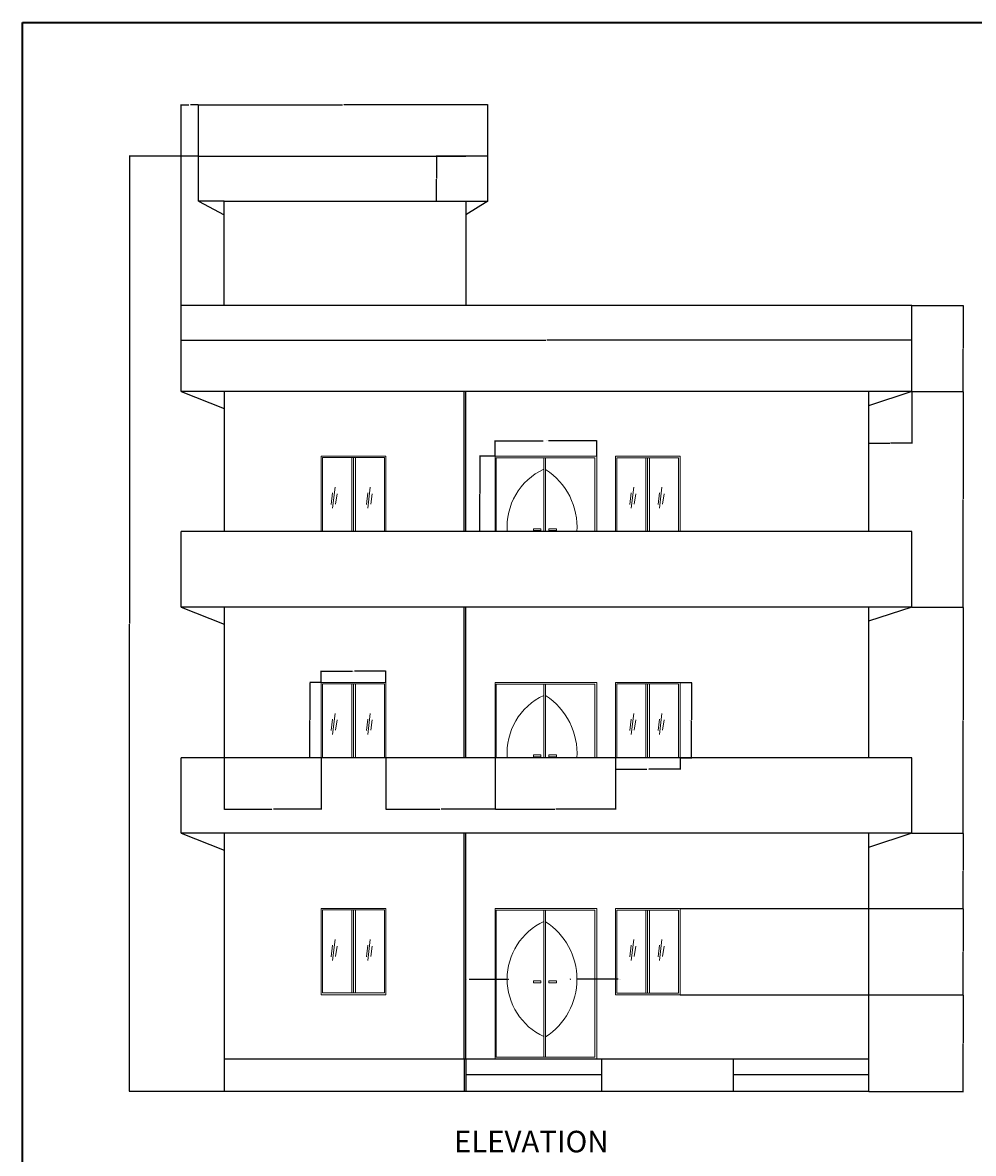
# Model space of a CAD drawing. Units: inches. Extents: x 1832 to 2989, y 1644 to 2902.
# Tile 7 of 8: x 1832 to 2361, y 2272 to 2902. Entities that reach past the tile are written whole.
import ezdxf

# ---------------------------------------------------------------- set-up
doc = ezdxf.new("R2010")
doc.units = ezdxf.units.IN
for name, color, linetype, lineweight in [('A-ANNO-DIMS', 2, 'Continuous', 18), ('A-ANNO-TEXT', 7, 'Continuous', 25), ('A-ANNO-TTLB', 7, 'Continuous', 35), ('A-ELEV', 7, 'Continuous', 25), ('A-ELEV-DOOR', 3, 'Continuous', 18), ('A-ELEV-GLAZ', 4, 'Continuous', 18)]:
    doc.layers.add(name, color=color, linetype=linetype, lineweight=lineweight)
doc.styles.get("Standard").update_dxf_attribs({"font": 'arial.ttf'})
doc.dimstyles.get("Standard").update_dxf_attribs({"dimtxt": 0.18, "dimasz": 0.18, "dimexe": 0.18, "dimexo": 0.0625, "dimgap": 0.09, "dimtad": 0, "dimtih": 1, "dimtoh": 1, "dimdec": 4, "dimzin": 0, "dimdsep": 46, "dimtxsty": 'Standard', "dimcen": 0.09, "dimadec": 0, "dimazin": 0, "dimtfac": 1, "dimtdec": 4, "dimtofl": 0, "dimtmove": 0, "dimatfit": 3, "dimfxl": 1, "dimtolj": 1, "dimtzin": 0, "dimarcsym": 0})

# ---------------------------------------------------------------- blocks, each defined once
blk = doc.blocks.new('WIN-ELEV-UPPER-LEFT')
for p, q in [((0, 42), (0, 0)), ((36, 42), (0, 42)), ((17.96, 41.22), (16.96, 41.22)), ((16.96, 41.22), (16.96, 0)), ((17.96, 41.22), (17.96, 0)), ((18.96, 41.22), (17.96, 41.22)), ((18.96, 0), (18.96, 41.22)), ((36, 42), (36, 0)), ((6.3, 21.56), (5.52, 15.16)), ((7.63, 24.74), (6.29, 13.04)), ((8.79, 21.07), (7.93, 15.34)), ((25.93, 21.56), (25.15, 15.16)), ((27.26, 24.74), (25.92, 13.04)), ((28.42, 21.07), (27.56, 15.34))]:
    blk.add_line(p, q)
blk.add_lwpolyline([(0.65, 0), (0.65, 41.22), (35.27, 41.22), (35.27, 0)])
blk = doc.blocks.new('DOOR-ELEV-UPPER')
for p, q in [((0, 42), (0, 0)), ((56.64, 42), (0, 42)), ((27.18, 0), (27.18, 41.04)), ((28.18, 41.04), (28.18, 0)), ((56.64, 42), (56.64, 0))]:
    blk.add_line(p, q)
blk.add_lwpolyline([(0.72, 0), (0.72, 41.04), (55.64, 41.04), (55.64, 0)])
for points in [[(21.46, 1.64), (25.62, 1.64), (25.62, 0.56), (21.46, 0.56)], [(30.06, 1.64), (34.22, 1.64), (34.22, 0.56), (30.06, 0.56)]]:
    blk.add_lwpolyline(points, close=True)
for centre, radius, start, end in [((42.11, 2.72), 35.37, 114.9672, 184.41429), ((7.59, 2.58), 38.09, 356.10922, 57.26734)]:
    blk.add_arc(centre, radius, start, end)
blk = doc.blocks.new('WIN-ELEV-UPPER-RIGHT')
for p, q in [((0, 42), (0, 0)), ((36, 42), (0, 42)), ((17.93, 41.14), (16.93, 41.14)), ((16.93, 41.14), (16.93, 0)), ((17.93, 41.14), (17.93, 0)), ((18.93, 0), (18.93, 41.14)), ((36, 42), (36, 0)), ((8.84, 21.56), (8.06, 15.16)), ((10.17, 24.74), (8.82, 13.04)), ((11.33, 21.07), (10.47, 15.34)), ((24.59, 21.56), (23.81, 15.16)), ((25.92, 24.74), (24.57, 13.04)), ((27.08, 21.07), (26.22, 15.34))]:
    blk.add_line(p, q)
blk.add_lwpolyline([(0.74, 0), (0.74, 41.14), (35.12, 41.14), (35.12, 0)])
blk = doc.blocks.new('*D61')
at = {"layer": 'A-ANNO-DIMS', "color": 0, "lineweight": -2, "transparency": 16777216}
for p, q in [((1997.98, 2534.31), (1991.56, 2534.31)), ((1991.74, 2534.13), (1991.74, 2513.5)), ((1991.74, 2492.49), (1991.74, 2513.13)), ((1997.98, 2492.31), (1991.56, 2492.31))]:
    blk.add_line(p, q, dxfattribs=at)
at = {"layer": 'A-ANNO-DIMS', "color": 0, "transparency": 16777216}
for points in [[(1991.71, 2534.13), (1991.77, 2534.13), (1991.74, 2534.31)], [(1991.71, 2492.49), (1991.77, 2492.49), (1991.74, 2492.31)]]:
    blk.add_solid(points, dxfattribs=at)
at = {"layer": 'Defpoints', "color": 0, "transparency": 16777216}
for p in [(1991.74, 2534.31), (1998.04, 2534.31), (1998.04, 2492.31)]:
    blk.add_point(p, dxfattribs=at)
at = {"layer": 'A-ANNO-DIMS', "color": 0, "transparency": 16777216, "insert": (1991.74, 2513.31), "char_height": 0.18, "attachment_point": 5}
blk.add_mtext('\\A1;LH WINDOW 42 TYP.', dxfattribs=at)
blk = doc.blocks.new('*D62')
at = {"layer": 'A-ANNO-DIMS', "color": 0, "lineweight": -2, "transparency": 16777216}
for p, q in [((1998.04, 2534.37), (1998.04, 2540.79)), ((1998.22, 2540.61), (2015.51, 2540.61)), ((2033.86, 2540.61), (2016.57, 2540.61)), ((2034.04, 2534.37), (2034.04, 2540.79))]:
    blk.add_line(p, q, dxfattribs=at)
at = {"layer": 'A-ANNO-DIMS', "color": 0, "transparency": 16777216}
for points in [[(1998.22, 2540.64), (1998.22, 2540.58), (1998.04, 2540.61)], [(2033.86, 2540.64), (2033.86, 2540.58), (2034.04, 2540.61)]]:
    blk.add_solid(points, dxfattribs=at)
at = {"layer": 'Defpoints', "color": 0, "transparency": 16777216}
for p in [(2034.04, 2540.61), (1998.04, 2534.31), (2034.04, 2534.31)]:
    blk.add_point(p, dxfattribs=at)
at = {"layer": 'A-ANNO-DIMS', "color": 0, "transparency": 16777216, "insert": (2016.04, 2540.61), "char_height": 0.18, "attachment_point": 5}
blk.add_mtext('\\A1;36 TYP.', dxfattribs=at)
blk = doc.blocks.new('*D63')
at = {"layer": 'A-ANNO-DIMS', "color": 0, "lineweight": -2, "transparency": 16777216}
for p, q in [((2094.8, 2660.37), (2094.8, 2668.99)), ((2094.98, 2668.81), (2121.71, 2668.81)), ((2151.25, 2668.81), (2124.52, 2668.81)), ((2151.43, 2660.37), (2151.43, 2668.99))]:
    blk.add_line(p, q, dxfattribs=at)
at = {"layer": 'A-ANNO-DIMS', "color": 0, "transparency": 16777216}
for points in [[(2094.98, 2668.84), (2094.98, 2668.78), (2094.8, 2668.81)], [(2151.25, 2668.84), (2151.25, 2668.78), (2151.43, 2668.81)]]:
    blk.add_solid(points, dxfattribs=at)
at = {"layer": 'Defpoints', "color": 0, "transparency": 16777216}
for p in [(2151.43, 2668.81), (2094.8, 2660.31), (2151.43, 2660.31)]:
    blk.add_point(p, dxfattribs=at)
at = {"layer": 'A-ANNO-DIMS', "color": 0, "transparency": 16777216, "insert": (2123.12, 2668.81), "char_height": 0.18, "attachment_point": 5}
blk.add_mtext('\\A1;UPPER DOOR 57 TYP.', dxfattribs=at)
blk = doc.blocks.new('*D64')
at = {"layer": 'A-ANNO-DIMS', "color": 0, "lineweight": -2, "transparency": 16777216}
for p, q in [((2094.73, 2660.31), (2086.12, 2660.31)), ((2086.3, 2660.13), (2086.3, 2639.49)), ((2086.3, 2618.49), (2086.3, 2639.13)), ((2094.73, 2618.31), (2086.12, 2618.31))]:
    blk.add_line(p, q, dxfattribs=at)
at = {"layer": 'A-ANNO-DIMS', "color": 0, "transparency": 16777216}
for points in [[(2086.27, 2660.13), (2086.33, 2660.13), (2086.3, 2660.31)], [(2086.27, 2618.49), (2086.33, 2618.49), (2086.3, 2618.31)]]:
    blk.add_solid(points, dxfattribs=at)
at = {"layer": 'Defpoints', "color": 0, "transparency": 16777216}
for p in [(2086.3, 2660.31), (2094.8, 2660.31), (2094.8, 2618.31)]:
    blk.add_point(p, dxfattribs=at)
at = {"layer": 'A-ANNO-DIMS', "color": 0, "transparency": 16777216, "insert": (2086.3, 2639.31), "char_height": 0.18, "attachment_point": 5}
blk.add_mtext('\\A1;42 TYP.', dxfattribs=at)
blk = doc.blocks.new('*D65')
at = {"layer": 'A-ANNO-DIMS', "color": 0, "lineweight": -2, "transparency": 16777216}
for p, q in [((2197.95, 2534.31), (2204.37, 2534.31)), ((2204.19, 2534.13), (2204.19, 2513.5)), ((2204.19, 2492.49), (2204.19, 2513.13)), ((2197.95, 2492.31), (2204.37, 2492.31))]:
    blk.add_line(p, q, dxfattribs=at)
at = {"layer": 'A-ANNO-DIMS', "color": 0, "transparency": 16777216}
for points in [[(2204.16, 2534.13), (2204.22, 2534.13), (2204.19, 2534.31)], [(2204.16, 2492.49), (2204.22, 2492.49), (2204.19, 2492.31)]]:
    blk.add_solid(points, dxfattribs=at)
at = {"layer": 'Defpoints', "color": 0, "transparency": 16777216}
for p in [(2197.89, 2534.31), (2204.19, 2534.31), (2197.89, 2492.31)]:
    blk.add_point(p, dxfattribs=at)
at = {"layer": 'A-ANNO-DIMS', "color": 0, "transparency": 16777216, "insert": (2204.19, 2513.31), "char_height": 0.18, "attachment_point": 5}
blk.add_mtext('\\A1;RH WINDOW 42 TYP.', dxfattribs=at)
blk = doc.blocks.new('*D66')
at = {"layer": 'A-ANNO-DIMS', "color": 0, "lineweight": -2, "transparency": 16777216}
for p, q in [((2161.89, 2492.25), (2161.89, 2485.83)), ((2197.89, 2492.25), (2197.89, 2485.83)), ((2162.07, 2486.01), (2179.36, 2486.01)), ((2197.71, 2486.01), (2180.42, 2486.01))]:
    blk.add_line(p, q, dxfattribs=at)
at = {"layer": 'A-ANNO-DIMS', "color": 0, "transparency": 16777216}
for points in [[(2162.07, 2486.04), (2162.07, 2485.98), (2161.89, 2486.01)], [(2197.71, 2486.04), (2197.71, 2485.98), (2197.89, 2486.01)]]:
    blk.add_solid(points, dxfattribs=at)
at = {"layer": 'Defpoints', "color": 0, "transparency": 16777216}
for p in [(2161.89, 2492.31), (2197.89, 2492.31), (2197.89, 2486.01)]:
    blk.add_point(p, dxfattribs=at)
at = {"layer": 'A-ANNO-DIMS', "color": 0, "transparency": 16777216, "insert": (2179.89, 2486.01), "char_height": 0.18, "attachment_point": 5}
blk.add_mtext('\\A1;36 TYP.', dxfattribs=at)
blk = doc.blocks.new('*D98')
at = {"layer": 'A-ANNO-DIMS', "color": 0, "lineweight": -2, "transparency": 16777216}
for p, q in [((1919.89, 2696.37), (1919.89, 2725.14)), ((1920.07, 2724.96), (2123.1, 2724.96)), ((2326.71, 2724.96), (2123.68, 2724.96)), ((2326.89, 2696.37), (2326.89, 2725.14))]:
    blk.add_line(p, q, dxfattribs=at)
at = {"layer": 'A-ANNO-DIMS', "color": 0, "transparency": 16777216}
for points in [[(1920.07, 2724.99), (1920.07, 2724.93), (1919.89, 2724.96)], [(2326.71, 2724.99), (2326.71, 2724.93), (2326.89, 2724.96)]]:
    blk.add_solid(points, dxfattribs=at)
at = {"layer": 'Defpoints', "color": 0, "transparency": 16777216}
for p in [(2326.89, 2724.96), (1919.89, 2696.31), (2326.89, 2696.31)]:
    blk.add_point(p, dxfattribs=at)
at = {"layer": 'A-ANNO-DIMS', "color": 0, "transparency": 16777216, "insert": (2123.39, 2724.96), "char_height": 0.18, "attachment_point": 5}
blk.add_mtext('\\A1;407', dxfattribs=at)
blk = doc.blocks.new('*D99')
at = {"layer": 'A-ANNO-DIMS', "color": 0, "lineweight": -2, "transparency": 16777216}
for p, q in [((1929.52, 2827.51), (1891.06, 2827.51)), ((1891.24, 2827.33), (1891.24, 2567.09)), ((1891.24, 2306.49), (1891.24, 2566.73)), ((1943.83, 2306.31), (1891.06, 2306.31))]:
    blk.add_line(p, q, dxfattribs=at)
at = {"layer": 'A-ANNO-DIMS', "color": 0, "transparency": 16777216}
for points in [[(1891.21, 2827.33), (1891.27, 2827.33), (1891.24, 2827.51)], [(1891.21, 2306.49), (1891.27, 2306.49), (1891.24, 2306.31)]]:
    blk.add_solid(points, dxfattribs=at)
at = {"layer": 'Defpoints', "color": 0, "transparency": 16777216}
for p in [(1891.24, 2827.51), (1929.58, 2827.51), (1943.89, 2306.31)]:
    blk.add_point(p, dxfattribs=at)
at = {"layer": 'A-ANNO-DIMS', "color": 0, "transparency": 16777216, "insert": (1891.24, 2566.91), "char_height": 0.18, "attachment_point": 5}
blk.add_mtext('\\A1;521.2', dxfattribs=at)
blk = doc.blocks.new('*D100')
at = {"layer": 'A-ANNO-DIMS', "color": 0, "lineweight": -2, "transparency": 16777216}
for p, q in [((1919.89, 2744.37), (1919.89, 2856.34)), ((1920.07, 2856.16), (1924.34, 2856.16)), ((1929.4, 2856.16), (1925.13, 2856.16)), ((1929.58, 2827.57), (1929.58, 2856.34))]:
    blk.add_line(p, q, dxfattribs=at)
at = {"layer": 'A-ANNO-DIMS', "color": 0, "transparency": 16777216}
for points in [[(1920.07, 2856.19), (1920.07, 2856.13), (1919.89, 2856.16)], [(1929.4, 2856.19), (1929.4, 2856.13), (1929.58, 2856.16)]]:
    blk.add_solid(points, dxfattribs=at)
at = {"layer": 'Defpoints', "color": 0, "transparency": 16777216}
for p in [(1929.58, 2856.16), (1929.58, 2827.51), (1919.89, 2744.31)]:
    blk.add_point(p, dxfattribs=at)
at = {"layer": 'A-ANNO-DIMS', "color": 0, "transparency": 16777216, "insert": (1924.74, 2856.16), "char_height": 0.18, "attachment_point": 5}
blk.add_mtext('\\A1;9.692', dxfattribs=at)
blk = doc.blocks.new('*D101')
at = {"layer": 'A-ANNO-DIMS', "color": 0, "lineweight": -2, "transparency": 16777216}
for p, q in [((1929.58, 2827.57), (1929.58, 2856.34)), ((1929.76, 2856.16), (2009.79, 2856.16)), ((2090.59, 2856.16), (2010.56, 2856.16)), ((2090.77, 2827.57), (2090.77, 2856.34))]:
    blk.add_line(p, q, dxfattribs=at)
at = {"layer": 'A-ANNO-DIMS', "color": 0, "transparency": 16777216}
for points in [[(1929.76, 2856.19), (1929.76, 2856.13), (1929.58, 2856.16)], [(2090.59, 2856.19), (2090.59, 2856.13), (2090.77, 2856.16)]]:
    blk.add_solid(points, dxfattribs=at)
at = {"layer": 'Defpoints', "color": 0, "transparency": 16777216}
for p in [(2090.77, 2856.16), (1929.58, 2827.51), (2090.77, 2827.51)]:
    blk.add_point(p, dxfattribs=at)
at = {"layer": 'A-ANNO-DIMS', "color": 0, "transparency": 16777216, "insert": (2010.18, 2856.16), "char_height": 0.18, "attachment_point": 5}
blk.add_mtext('\\A1;161.2', dxfattribs=at)
blk = doc.blocks.new('*D102')
at = {"layer": 'A-ANNO-DIMS', "color": 0, "lineweight": -2, "transparency": 16777216}
for p, q in [((2302.89, 2696.25), (2302.89, 2667.48)), ((2326.89, 2696.25), (2326.89, 2667.48)), ((2303.07, 2667.66), (2314.67, 2667.66)), ((2326.71, 2667.66), (2315.11, 2667.66))]:
    blk.add_line(p, q, dxfattribs=at)
at = {"layer": 'A-ANNO-DIMS', "color": 0, "transparency": 16777216}
for points in [[(2303.07, 2667.69), (2303.07, 2667.63), (2302.89, 2667.66)], [(2326.71, 2667.69), (2326.71, 2667.63), (2326.89, 2667.66)]]:
    blk.add_solid(points, dxfattribs=at)
at = {"layer": 'Defpoints', "color": 0, "transparency": 16777216}
for p in [(2302.89, 2696.31), (2326.89, 2696.31), (2302.89, 2667.66)]:
    blk.add_point(p, dxfattribs=at)
at = {"layer": 'A-ANNO-DIMS', "color": 0, "transparency": 16777216, "insert": (2314.89, 2667.66), "char_height": 0.18, "attachment_point": 5}
blk.add_mtext('\\A1;24', dxfattribs=at)
blk = doc.blocks.new('*D103')
at = {"layer": 'A-ANNO-DIMS', "color": 0, "lineweight": -2, "transparency": 16777216}
for p, q in [((2197.95, 2360.31), (2355.72, 2360.31)), ((2355.54, 2360.13), (2355.54, 2333.49)), ((2355.54, 2306.49), (2355.54, 2333.13)), ((2302.95, 2306.31), (2355.72, 2306.31))]:
    blk.add_line(p, q, dxfattribs=at)
at = {"layer": 'A-ANNO-DIMS', "color": 0, "transparency": 16777216}
for points in [[(2355.51, 2360.13), (2355.57, 2360.13), (2355.54, 2360.31)], [(2355.51, 2306.49), (2355.57, 2306.49), (2355.54, 2306.31)]]:
    blk.add_solid(points, dxfattribs=at)
at = {"layer": 'Defpoints', "color": 0, "transparency": 16777216}
for p in [(2197.89, 2360.31), (2355.54, 2360.31), (2302.89, 2306.31)]:
    blk.add_point(p, dxfattribs=at)
at = {"layer": 'A-ANNO-DIMS', "color": 0, "transparency": 16777216, "insert": (2355.54, 2333.31), "char_height": 0.18, "attachment_point": 5}
blk.add_mtext('\\A1;54', dxfattribs=at)
blk = doc.blocks.new('*D104')
at = {"layer": 'A-ANNO-DIMS', "color": 0, "lineweight": -2, "transparency": 16777216}
for p, q in [((2197.95, 2408.31), (2355.72, 2408.31)), ((2355.54, 2408.13), (2355.54, 2384.49)), ((2355.54, 2360.49), (2355.54, 2384.13)), ((2197.95, 2360.31), (2355.72, 2360.31))]:
    blk.add_line(p, q, dxfattribs=at)
at = {"layer": 'A-ANNO-DIMS', "color": 0, "transparency": 16777216}
for points in [[(2355.51, 2408.13), (2355.57, 2408.13), (2355.54, 2408.31)], [(2355.51, 2360.49), (2355.57, 2360.49), (2355.54, 2360.31)]]:
    blk.add_solid(points, dxfattribs=at)
at = {"layer": 'Defpoints', "color": 0, "transparency": 16777216}
for p in [(2197.89, 2408.31), (2355.54, 2408.31), (2197.89, 2360.31)]:
    blk.add_point(p, dxfattribs=at)
at = {"layer": 'A-ANNO-DIMS', "color": 0, "transparency": 16777216, "insert": (2355.54, 2384.31), "char_height": 0.18, "attachment_point": 5}
blk.add_mtext('\\A1;48', dxfattribs=at)
blk = doc.blocks.new('*D105')
at = {"layer": 'A-ANNO-DIMS', "color": 0, "lineweight": -2, "transparency": 16777216}
for p, q in [((2326.95, 2450.31), (2355.72, 2450.31)), ((2355.54, 2450.13), (2355.54, 2429.49)), ((2355.54, 2408.49), (2355.54, 2429.13)), ((2197.95, 2408.31), (2355.72, 2408.31))]:
    blk.add_line(p, q, dxfattribs=at)
at = {"layer": 'A-ANNO-DIMS', "color": 0, "transparency": 16777216}
for points in [[(2355.51, 2450.13), (2355.57, 2450.13), (2355.54, 2450.31)], [(2355.51, 2408.49), (2355.57, 2408.49), (2355.54, 2408.31)]]:
    blk.add_solid(points, dxfattribs=at)
at = {"layer": 'Defpoints', "color": 0, "transparency": 16777216}
for p in [(2326.89, 2450.31), (2355.54, 2450.31), (2197.89, 2408.31)]:
    blk.add_point(p, dxfattribs=at)
at = {"layer": 'A-ANNO-DIMS', "color": 0, "transparency": 16777216, "insert": (2355.54, 2429.31), "char_height": 0.18, "attachment_point": 5}
blk.add_mtext('\\A1;42', dxfattribs=at)
blk = doc.blocks.new('*D106')
at = {"layer": 'A-ANNO-DIMS', "color": 0, "lineweight": -2, "transparency": 16777216}
for p, q in [((2326.95, 2576.31), (2355.72, 2576.31)), ((2355.54, 2576.13), (2355.54, 2513.49)), ((2355.54, 2450.49), (2355.54, 2513.13)), ((2326.95, 2450.31), (2355.72, 2450.31))]:
    blk.add_line(p, q, dxfattribs=at)
at = {"layer": 'A-ANNO-DIMS', "color": 0, "transparency": 16777216}
for points in [[(2355.51, 2576.13), (2355.57, 2576.13), (2355.54, 2576.31)], [(2355.51, 2450.49), (2355.57, 2450.49), (2355.54, 2450.31)]]:
    blk.add_solid(points, dxfattribs=at)
at = {"layer": 'Defpoints', "color": 0, "transparency": 16777216}
for p in [(2326.89, 2576.31), (2355.54, 2576.31), (2326.89, 2450.31)]:
    blk.add_point(p, dxfattribs=at)
at = {"layer": 'A-ANNO-DIMS', "color": 0, "transparency": 16777216, "insert": (2355.54, 2513.31), "char_height": 0.18, "attachment_point": 5}
blk.add_mtext('\\A1;126', dxfattribs=at)
blk = doc.blocks.new('*D107')
at = {"layer": 'A-ANNO-DIMS', "color": 0, "lineweight": -2, "transparency": 16777216}
for p, q in [((2326.95, 2696.31), (2355.72, 2696.31)), ((2355.54, 2696.13), (2355.54, 2636.49)), ((2355.54, 2576.49), (2355.54, 2636.13)), ((2326.95, 2576.31), (2355.72, 2576.31))]:
    blk.add_line(p, q, dxfattribs=at)
at = {"layer": 'A-ANNO-DIMS', "color": 0, "transparency": 16777216}
for points in [[(2355.51, 2696.13), (2355.57, 2696.13), (2355.54, 2696.31)], [(2355.51, 2576.49), (2355.57, 2576.49), (2355.54, 2576.31)]]:
    blk.add_solid(points, dxfattribs=at)
at = {"layer": 'Defpoints', "color": 0, "transparency": 16777216}
for p in [(2326.89, 2696.31), (2355.54, 2696.31), (2326.89, 2576.31)]:
    blk.add_point(p, dxfattribs=at)
at = {"layer": 'A-ANNO-DIMS', "color": 0, "transparency": 16777216, "insert": (2355.54, 2636.31), "char_height": 0.18, "attachment_point": 5}
blk.add_mtext('\\A1;120', dxfattribs=at)
blk = doc.blocks.new('*D108')
at = {"layer": 'A-ANNO-DIMS', "color": 0, "lineweight": -2, "transparency": 16777216}
for p, q in [((2326.95, 2744.31), (2355.72, 2744.31)), ((2355.54, 2744.13), (2355.54, 2720.49)), ((2355.54, 2696.49), (2355.54, 2720.13)), ((2326.95, 2696.31), (2355.72, 2696.31))]:
    blk.add_line(p, q, dxfattribs=at)
at = {"layer": 'A-ANNO-DIMS', "color": 0, "transparency": 16777216}
for points in [[(2355.51, 2744.13), (2355.57, 2744.13), (2355.54, 2744.31)], [(2355.51, 2696.49), (2355.57, 2696.49), (2355.54, 2696.31)]]:
    blk.add_solid(points, dxfattribs=at)
at = {"layer": 'Defpoints', "color": 0, "transparency": 16777216}
for p in [(2326.89, 2744.31), (2355.54, 2744.31), (2326.89, 2696.31)]:
    blk.add_point(p, dxfattribs=at)
at = {"layer": 'A-ANNO-DIMS', "color": 0, "transparency": 16777216, "insert": (2355.54, 2720.31), "char_height": 0.18, "attachment_point": 5}
blk.add_mtext('\\A1;48', dxfattribs=at)
blk = doc.blocks.new('*D109')
at = {"layer": 'A-ANNO-DIMS', "color": 0, "lineweight": -2, "transparency": 16777216}
for p, q in [((2090.71, 2827.51), (2061.94, 2827.51)), ((2062.12, 2827.33), (2062.12, 2815.1)), ((2062.12, 2802.51), (2062.12, 2814.74)), ((2090.71, 2802.33), (2061.94, 2802.33))]:
    blk.add_line(p, q, dxfattribs=at)
at = {"layer": 'A-ANNO-DIMS', "color": 0, "transparency": 16777216}
for points in [[(2062.09, 2827.33), (2062.15, 2827.33), (2062.12, 2827.51)], [(2062.09, 2802.51), (2062.15, 2802.51), (2062.12, 2802.33)]]:
    blk.add_solid(points, dxfattribs=at)
at = {"layer": 'Defpoints', "color": 0, "transparency": 16777216}
for p in [(2062.12, 2827.51), (2090.77, 2827.51), (2090.77, 2802.33)]:
    blk.add_point(p, dxfattribs=at)
at = {"layer": 'A-ANNO-DIMS', "color": 0, "transparency": 16777216, "insert": (2062.12, 2814.92), "char_height": 0.18, "attachment_point": 5}
blk.add_mtext('\\A1;25.175', dxfattribs=at)
blk = doc.blocks.new('*D110')
at = {"layer": 'A-ANNO-DIMS', "color": 0, "lineweight": -2, "transparency": 16777216}
for p, q in [((1943.89, 2492.25), (1943.89, 2463.48)), ((1998.04, 2492.25), (1998.04, 2463.48)), ((1944.07, 2463.66), (1970.57, 2463.66)), ((1997.86, 2463.66), (1971.36, 2463.66))]:
    blk.add_line(p, q, dxfattribs=at)
at = {"layer": 'A-ANNO-DIMS', "color": 0, "transparency": 16777216}
for points in [[(1944.07, 2463.69), (1944.07, 2463.63), (1943.89, 2463.66)], [(1997.86, 2463.69), (1997.86, 2463.63), (1998.04, 2463.66)]]:
    blk.add_solid(points, dxfattribs=at)
at = {"layer": 'Defpoints', "color": 0, "transparency": 16777216}
for p in [(1943.89, 2492.31), (1998.04, 2492.31), (1943.89, 2463.66)]:
    blk.add_point(p, dxfattribs=at)
at = {"layer": 'A-ANNO-DIMS', "color": 0, "transparency": 16777216, "insert": (1970.97, 2463.66), "char_height": 0.18, "attachment_point": 5}
blk.add_mtext('\\A1;54.15', dxfattribs=at)
blk = doc.blocks.new('*D111')
at = {"layer": 'A-ANNO-DIMS', "color": 0, "lineweight": -2, "transparency": 16777216}
for p, q in [((2034.04, 2492.25), (2034.04, 2463.48)), ((2094.8, 2492.25), (2094.8, 2463.48)), ((2034.22, 2463.66), (2064.02, 2463.66)), ((2094.62, 2463.66), (2064.81, 2463.66))]:
    blk.add_line(p, q, dxfattribs=at)
at = {"layer": 'A-ANNO-DIMS', "color": 0, "transparency": 16777216}
for points in [[(2034.22, 2463.69), (2034.22, 2463.63), (2034.04, 2463.66)], [(2094.62, 2463.69), (2094.62, 2463.63), (2094.8, 2463.66)]]:
    blk.add_solid(points, dxfattribs=at)
at = {"layer": 'Defpoints', "color": 0, "transparency": 16777216}
for p in [(2034.04, 2492.31), (2094.8, 2492.31), (2034.04, 2463.66)]:
    blk.add_point(p, dxfattribs=at)
at = {"layer": 'A-ANNO-DIMS', "color": 0, "transparency": 16777216, "insert": (2064.42, 2463.66), "char_height": 0.18, "attachment_point": 5}
blk.add_mtext('\\A1;60.76', dxfattribs=at)
blk = doc.blocks.new('*D112')
at = {"layer": 'A-ANNO-DIMS', "color": 0, "lineweight": -2, "transparency": 16777216}
for p, q in [((2094.8, 2492.25), (2094.8, 2463.48)), ((2161.89, 2492.25), (2161.89, 2463.48)), ((2094.98, 2463.66), (2128.04, 2463.66)), ((2161.71, 2463.66), (2128.65, 2463.66))]:
    blk.add_line(p, q, dxfattribs=at)
at = {"layer": 'A-ANNO-DIMS', "color": 0, "transparency": 16777216}
for points in [[(2094.98, 2463.69), (2094.98, 2463.63), (2094.8, 2463.66)], [(2161.71, 2463.69), (2161.71, 2463.63), (2161.89, 2463.66)]]:
    blk.add_solid(points, dxfattribs=at)
at = {"layer": 'Defpoints', "color": 0, "transparency": 16777216}
for p in [(2094.8, 2492.31), (2161.89, 2492.31), (2094.8, 2463.66)]:
    blk.add_point(p, dxfattribs=at)
at = {"layer": 'A-ANNO-DIMS', "color": 0, "transparency": 16777216, "insert": (2128.34, 2463.66), "char_height": 0.18, "attachment_point": 5}
blk.add_mtext('\\A1;67.1', dxfattribs=at)
blk = doc.blocks.new('*D128')
at = {"layer": 'A-ANNO-DIMS', "color": 0, "lineweight": -2, "transparency": 16777216}
for p, q in [((2102.29, 2368.9), (2102.47, 2368.9)), ((2102.38, 2368.81), (2102.38, 2368.99)), ((2163.32, 2368.9), (2140.65, 2368.9))]:
    blk.add_line(p, q, dxfattribs=at)
at = {"layer": 'A-ANNO-DIMS', "color": 0, "transparency": 16777216}
blk.add_solid([(2140.65, 2368.93), (2140.65, 2368.87), (2140.47, 2368.9)], dxfattribs=at)
at = {"layer": 'Defpoints', "color": 0, "transparency": 16777216}
for p in [(2102.38, 2368.9), (2140.47, 2368.9)]:
    blk.add_point(p, dxfattribs=at)
at = {"layer": 'A-ANNO-DIMS', "color": 0, "transparency": 16777216, "insert": (2164.06, 2368.9), "char_height": 0.18, "attachment_point": 5}
blk.add_mtext('\\A1;3X R38.086', dxfattribs=at)
blk = doc.blocks.new('*D129')
at = {"layer": 'A-ANNO-DIMS', "color": 0, "lineweight": -2, "transparency": 16777216}
for p, q in [((2080.32, 2369.03), (2101.36, 2369.03)), ((2136.81, 2369.03), (2136.99, 2369.03)), ((2136.9, 2368.94), (2136.9, 2369.12))]:
    blk.add_line(p, q, dxfattribs=at)
at = {"layer": 'A-ANNO-DIMS', "color": 0, "transparency": 16777216}
blk.add_solid([(2101.36, 2369.06), (2101.36, 2369), (2101.54, 2369.03)], dxfattribs=at)
at = {"layer": 'Defpoints', "color": 0, "transparency": 16777216}
for p in [(2101.54, 2369.03), (2136.9, 2369.03)]:
    blk.add_point(p, dxfattribs=at)
at = {"layer": 'A-ANNO-DIMS', "color": 0, "transparency": 16777216, "insert": (2079.64, 2369.03), "char_height": 0.18, "attachment_point": 5}
blk.add_mtext('\\A1;3X R35.37', dxfattribs=at)

msp = doc.modelspace()

# ---------------------------------------------------------------- linework, layer by layer
at = {"layer": 'A-ANNO-TTLB'}
msp.add_lwpolyline([(1831.6677, 2901.9044), (2988.9144, 2901.9044), (2988.9144, 1643.5851), (1831.6677, 1643.5851)], close=True, dxfattribs=at)
at = {"layer": 'A-ELEV'}
for p, q in [((1929.5824, 2802.3343), (1929.5824, 2827.509)), ((1929.5824, 2827.509), (1943.8904, 2827.509)), ((1943.8904, 2827.509), (2078.5865, 2827.509)), ((2078.5865, 2827.509), (2078.5865, 2827.509)), ((2090.7705, 2827.509), (2078.5865, 2827.509)), ((2090.7705, 2802.3343), (2090.7705, 2827.509)), ((1943.8904, 2802.3343), (1929.5824, 2802.3343)), ((1929.5824, 2802.3343), (1943.8904, 2794.7432)), ((1943.8904, 2744.3121), (1943.8904, 2802.3343)), ((1943.8904, 2802.3343), (2078.5865, 2802.3343)), ((2078.5865, 2802.3343), (2078.5865, 2744.3121)), ((2078.5865, 2802.3343), (2090.7705, 2802.3343)), ((2090.7705, 2802.3343), (2078.5865, 2794.7847)), ((2326.8904, 2744.3121), (1919.8904, 2744.3121)), ((1919.8904, 2696.3121), (1919.8904, 2744.3121)), ((2326.8904, 2696.3121), (2326.8904, 2744.3121)), ((2326.8904, 2696.3121), (1919.8904, 2696.3121)), ((1919.8904, 2696.3121), (1943.8904, 2686.8418)), ((1943.8904, 2696.3121), (1943.8904, 2618.3121)), ((2077.5865, 2618.3121), (2077.5865, 2696.3121)), ((2078.5865, 2618.3121), (2078.5865, 2696.3121)), ((2302.8904, 2696.3121), (2302.8904, 2618.3121)), ((2326.8904, 2696.3121), (2302.8904, 2688.3321)), ((2326.8904, 2618.3121), (1919.8904, 2618.3121)), ((2326.8904, 2618.3121), (1919.8904, 2618.3121)), ((1919.8904, 2576.3121), (1919.8904, 2618.3121)), ((2326.8904, 2576.3121), (2326.8904, 2618.3121)), ((2326.8904, 2576.3121), (1919.8904, 2576.3121)), ((2326.8904, 2576.3121), (1919.8904, 2576.3121)), ((1919.8904, 2576.3121), (1943.8904, 2566.8418)), ((1943.8904, 2576.3121), (1943.8904, 2492.3121)), ((1943.8904, 2576.3121), (1943.8904, 2492.3121)), ((1943.8904, 2576.3121), (1943.8904, 2558.3121)), ((2077.5865, 2492.3121), (2077.5865, 2576.3121)), ((2078.5865, 2492.3121), (2078.5865, 2576.3121)), ((2078.5865, 2492.3121), (2078.5865, 2576.3121)), ((2302.8904, 2576.3121), (2302.8904, 2492.3121)), ((2302.8904, 2576.3121), (2302.8904, 2492.3121)), ((2302.8904, 2576.3121), (2302.8904, 2558.3121)), ((2326.8904, 2576.3121), (2302.8904, 2568.3321)), ((2326.8904, 2492.3121), (1919.8904, 2492.3121)), ((1919.8904, 2450.3121), (1919.8904, 2492.3121)), ((2326.8904, 2450.3121), (2326.8904, 2492.3121)), ((2326.8904, 2450.3121), (1919.8904, 2450.3121)), ((1919.8904, 2450.3121), (1943.8904, 2440.8418)), ((1943.8904, 2450.3121), (1943.8904, 2306.3121)), ((1943.8904, 2450.3121), (1943.8904, 2432.3121)), ((1943.8904, 2450.3121), (1943.8904, 2432.3121)), ((2077.5865, 2324.3121), (2077.5865, 2450.3121)), ((2078.5865, 2324.3121), (2078.5865, 2450.3121)), ((2302.8904, 2450.3121), (2302.8904, 2306.3121)), ((2302.8904, 2450.3121), (2302.8904, 2432.3121)), ((2326.8904, 2450.3121), (2302.8904, 2442.3321)), ((2302.8904, 2324.3121), (1943.8904, 2324.3121)), ((2078.5865, 2324.3121), (2077.5865, 2324.3121)), ((2077.5865, 2324.3121), (2077.5865, 2306.3121)), ((2078.5865, 2324.3121), (2078.5865, 2306.3121)), ((2154.3769, 2306.3121), (2154.3769, 2324.3121)), ((2227.639, 2306.3121), (2227.639, 2324.3121)), ((2154.3769, 2315.5759), (2078.5865, 2315.5759)), ((2302.8904, 2315.5759), (2227.639, 2315.5759)), ((2302.8904, 2306.3121), (1943.8904, 2306.3121))]:
    msp.add_line(p, q, dxfattribs=at)
at = {"layer": 'A-ELEV-DOOR'}
for p, q in [((2094.7965, 2660.3121), (2094.7965, 2618.3121)), ((2151.4347, 2660.3121), (2094.7965, 2660.3121)), ((2151.4347, 2660.3121), (2151.4347, 2618.3121)), ((2094.7965, 2534.3121), (2094.7965, 2492.3121)), ((2151.4347, 2534.3121), (2094.7965, 2534.3121)), ((2094.7965, 2534.3121), (2094.7965, 2492.3121)), ((2151.4347, 2534.3121), (2094.7965, 2534.3121)), ((2151.4347, 2534.3121), (2151.4347, 2492.3121)), ((2151.4347, 2534.3121), (2151.4347, 2492.3121)), ((2094.7965, 2408.3121), (2094.7965, 2324.3121)), ((2151.4347, 2408.3121), (2094.7965, 2408.3121)), ((2121.9753, 2325.4737), (2121.9753, 2407.3475)), ((2122.9753, 2407.3475), (2122.9753, 2325.4737)), ((2151.4347, 2408.3121), (2151.4347, 2324.3121)), ((2122.9753, 2325.4737), (2121.9753, 2325.4737))]:
    msp.add_line(p, q, dxfattribs=at)
for points in [[(2095.5154, 2407.3475), (2150.4351, 2407.3475), (2150.4351, 2325.4737), (2095.5154, 2325.4737)], [(2116.2566, 2367.957), (2120.415, 2367.957), (2120.415, 2366.871), (2116.2566, 2366.871)], [(2124.8549, 2367.957), (2129.0133, 2367.957), (2129.0133, 2366.871), (2124.8549, 2366.871)]]:
    msp.add_lwpolyline(points, close=True, dxfattribs=at)
for centre, radius, start, end in [((2136.9035, 2369.0342), 35.3666, 114.9671951, 245.0328049), ((2102.3815, 2368.8964), 38.0859, 302.7326593, 57.2673407)]:
    msp.add_arc(centre, radius, start, end, dxfattribs=at)
at = {"layer": 'A-ELEV-GLAZ'}
for p, q in [((1998.0413, 2660.3121), (1998.0413, 2618.3121)), ((2034.0413, 2660.3121), (1998.0413, 2660.3121)), ((2034.0413, 2660.3121), (2034.0413, 2618.3121)), ((2161.8904, 2660.3121), (2161.8904, 2618.3121)), ((2197.8904, 2660.3121), (2161.8904, 2660.3121)), ((2197.8904, 2660.3121), (2197.8904, 2618.3121)), ((1998.0413, 2534.3121), (1998.0413, 2492.3121)), ((2034.0413, 2534.3121), (1998.0413, 2534.3121)), ((1998.0413, 2534.3121), (1998.0413, 2492.3121)), ((2034.0413, 2534.3121), (1998.0413, 2534.3121)), ((2034.0413, 2534.3121), (2034.0413, 2492.3121)), ((2034.0413, 2534.3121), (2034.0413, 2492.3121)), ((2161.8904, 2534.3121), (2161.8904, 2492.3121)), ((2197.8904, 2534.3121), (2161.8904, 2534.3121)), ((2161.8904, 2534.3121), (2161.8904, 2492.3121)), ((2197.8904, 2534.3121), (2161.8904, 2534.3121)), ((2197.8904, 2534.3121), (2197.8904, 2492.3121)), ((2197.8904, 2534.3121), (2197.8904, 2492.3121)), ((1998.0413, 2408.3121), (1998.0413, 2360.3121)), ((2034.0413, 2408.3121), (1998.0413, 2408.3121)), ((2016.0011, 2407.5335), (2015.0011, 2407.5335)), ((2015.0011, 2407.5335), (2015.0011, 2361.3035)), ((2016.0011, 2407.5335), (2016.0011, 2361.3035)), ((2017.0011, 2407.5335), (2016.0011, 2407.5335)), ((2017.0011, 2361.3035), (2017.0011, 2407.5335)), ((2034.0413, 2408.3121), (2034.0413, 2360.3121)), ((2161.8904, 2408.3121), (2161.8904, 2360.3121)), ((2197.8904, 2408.3121), (2161.8904, 2408.3121)), ((2179.8223, 2407.4521), (2178.8223, 2407.4521)), ((2178.8223, 2407.4521), (2178.8223, 2361.1625)), ((2179.8223, 2407.4521), (2179.8223, 2361.1625)), ((2180.8223, 2361.1625), (2180.8223, 2407.4521)), ((2197.8904, 2408.3121), (2197.8904, 2360.3121)), ((2004.3412, 2387.8755), (2003.5651, 2381.4712)), ((2005.6724, 2391.0493), (2004.3273, 2379.3519)), ((2023.9715, 2387.8755), (2023.1954, 2381.4712)), ((2025.3027, 2391.0493), (2023.9577, 2379.3519)), ((2170.7278, 2387.8755), (2169.9517, 2381.4712)), ((2172.059, 2391.0493), (2170.7139, 2379.3519)), ((2186.476, 2387.8755), (2185.6999, 2381.4712)), ((2187.8072, 2391.0493), (2186.4621, 2379.3519)), ((2006.8346, 2387.3803), (2005.9759, 2381.6527)), ((2026.465, 2387.3803), (2025.6063, 2381.6527)), ((2173.2212, 2387.3803), (2172.3625, 2381.6527)), ((2188.9694, 2387.3803), (2188.1108, 2381.6527)), ((2034.0413, 2360.3121), (1998.0413, 2360.3121)), ((2016.0011, 2361.3035), (2017.0011, 2361.3035)), ((2197.8904, 2360.3121), (2161.8904, 2360.3121)), ((2178.8223, 2361.1625), (2179.8223, 2361.1625)), ((2179.8223, 2361.1625), (2180.8223, 2361.1625))]:
    msp.add_line(p, q, dxfattribs=at)
for points in [[(1998.6927, 2407.5335), (2033.3095, 2407.5335), (2033.3095, 2361.3035), (1998.6927, 2361.3035)], [(2162.6309, 2407.4521), (2197.0137, 2407.4521), (2197.0137, 2361.1625), (2162.6309, 2361.1625)]]:
    msp.add_lwpolyline(points, close=True, dxfattribs=at)

# ---------------------------------------------------------------- block references
at = {"layer": 'A-ELEV-DOOR'}
for p in [(2094.7965, 2618.3121), (2094.7965, 2492.3121)]:
    msp.add_blockref('DOOR-ELEV-UPPER', p, dxfattribs=at)
at = {"layer": 'A-ELEV-GLAZ'}
for name, p in [('WIN-ELEV-UPPER-LEFT', (1998.0413, 2618.3121)), ('WIN-ELEV-UPPER-RIGHT', (2161.8904, 2618.3121)), ('WIN-ELEV-UPPER-LEFT', (1998.0413, 2492.3121)), ('WIN-ELEV-UPPER-RIGHT', (2161.8904, 2492.3121))]:
    msp.add_blockref(name, p, dxfattribs=at)

# ---------------------------------------------------------------- texts
at = {"layer": 'A-ANNO-TEXT', "insert": (2071.9161, 2284.4812), "char_height": 12, "attachment_point": 1}
msp.add_mtext_dynamic_manual_height_columns('ELEVATION', width=248.781202, gutter_width=12.5, heights=[0], dxfattribs=at)

# ---------------------------------------------------------------- dimensions: what is measured, and where the dimension line sits
at = {"layer": 'A-ANNO-DIMS'}
for base, p1, p2, override, picture, middle in [((1929.5824, 2856.159), (1919.8904, 2744.3121), (1929.5824, 2827.509), {"dimdec": 3, "dimlfac": 1, "dimrnd": 0, "dimzin": 0, "dimdsep": 46, "dimlunit": 2}, '*D100', (1924.7364, 2856.159)), ((2090.7705, 2856.159), (1929.5824, 2827.509), (2090.7705, 2827.509), {"dimdec": 1, "dimlfac": 1, "dimrnd": 0, "dimzin": 0, "dimdsep": 46, "dimlunit": 2}, '*D101', (2010.1765, 2856.159)), ((2326.8904, 2724.9621), (1919.8904, 2696.3121), (2326.8904, 2696.3121), {"dimdec": 0, "dimlfac": 1, "dimrnd": 0, "dimzin": 0, "dimdsep": 46, "dimlunit": 2}, '*D98', (2123.3904, 2724.9621))]:
    dim = msp.add_linear_dim(base=base, p1=p1, p2=p2, dimstyle='Standard', override=override, dxfattribs=at)
    dim.commit()
    dim.dimension.update_dxf_attribs({"geometry": picture, "text_midpoint": middle})
for base, p1, p2, angle, override, picture, middle in [((1891.2404, 2827.509), (1943.8904, 2306.3121), (1929.5824, 2827.509), 90, {"dimdec": 1, "dimlfac": 1, "dimrnd": 0, "dimzin": 0, "dimdsep": 46, "dimlunit": 2}, '*D99', (1891.2404, 2566.9105)), ((2062.1205, 2827.509), (2090.7705, 2802.3343), (2090.7705, 2827.509), 90, {"dimdec": 3, "dimlfac": 1, "dimrnd": 0, "dimzin": 0, "dimdsep": 46, "dimlunit": 2}, '*D109', (2062.1205, 2814.9216)), ((2355.5404, 2744.3121), (2326.8904, 2696.3121), (2326.8904, 2744.3121), 90, {"dimdec": 0, "dimlfac": 1, "dimrnd": 0, "dimzin": 0, "dimdsep": 46, "dimlunit": 2}, '*D108', (2355.5404, 2720.3121)), ((2302.8904, 2667.6621), (2326.8904, 2696.3121), (2302.8904, 2696.3121), 180, {"dimdec": 0, "dimlfac": 1, "dimrnd": 0, "dimzin": 0, "dimdsep": 46, "dimlunit": 2}, '*D102', (2314.8904, 2667.6621)), ((2355.5404, 2696.3121), (2326.8904, 2576.3121), (2326.8904, 2696.3121), 90, {"dimdec": 0, "dimlfac": 1, "dimrnd": 0, "dimzin": 0, "dimdsep": 46, "dimlunit": 2}, '*D107', (2355.5404, 2636.3121)), ((2355.5404, 2576.3121), (2326.8904, 2450.3121), (2326.8904, 2576.3121), 90, {"dimdec": 0, "dimlfac": 1, "dimrnd": 0, "dimzin": 0, "dimdsep": 46, "dimlunit": 2}, '*D106', (2355.5404, 2513.3121)), ((1943.8904, 2463.6621), (1998.0413, 2492.3121), (1943.8904, 2492.3121), 180, {"dimdec": 2, "dimlfac": 1, "dimrnd": 0, "dimzin": 0, "dimdsep": 46, "dimlunit": 2}, '*D110', (1970.9659, 2463.6621)), ((2034.0413, 2463.6621), (2094.7965, 2492.3121), (2034.0413, 2492.3121), 180, {"dimdec": 2, "dimlfac": 1, "dimrnd": 0, "dimzin": 0, "dimdsep": 46, "dimlunit": 2}, '*D111', (2064.4189, 2463.6621)), ((2094.7965, 2463.6621), (2161.8904, 2492.3121), (2094.7965, 2492.3121), 180, {"dimdec": 1, "dimlfac": 1, "dimrnd": 0, "dimzin": 0, "dimdsep": 46, "dimlunit": 2}, '*D112', (2128.3434, 2463.6621)), ((2355.5404, 2450.3121), (2197.8904, 2408.3121), (2326.8904, 2450.3121), 90, {"dimdec": 0, "dimlfac": 1, "dimrnd": 0, "dimzin": 0, "dimdsep": 46, "dimlunit": 2}, '*D105', (2355.5404, 2429.3121)), ((2355.5404, 2408.3121), (2197.8904, 2360.3121), (2197.8904, 2408.3121), 90, {"dimdec": 0, "dimlfac": 1, "dimrnd": 0, "dimzin": 0, "dimdsep": 46, "dimlunit": 2}, '*D104', (2355.5404, 2384.3121)), ((2355.5404, 2360.3121), (2302.8904, 2306.3121), (2197.8904, 2360.3121), 90, {"dimdec": 0, "dimlfac": 1, "dimrnd": 0, "dimzin": 0, "dimdsep": 46, "dimlunit": 2}, '*D103', (2355.5404, 2333.3121))]:
    dim = msp.add_linear_dim(base=base, p1=p1, p2=p2, angle=angle, dimstyle='Standard', override=override, dxfattribs=at)
    dim.commit()
    dim.dimension.update_dxf_attribs({"geometry": picture, "text_midpoint": middle})
for base, p1, p2, text, picture, middle in [((2151.4347, 2668.8078), (2094.7965, 2660.3121), (2151.4347, 2660.3121), 'UPPER DOOR <> TYP.', '*D63', (2123.1156, 2668.8078)), ((2034.0413, 2540.6121), (1998.0413, 2534.3121), (2034.0413, 2534.3121), '<> TYP.', '*D62', (2016.0413, 2540.6121)), ((2197.8904, 2486.0121), (2161.8904, 2492.3121), (2197.8904, 2492.3121), '<> TYP.', '*D66', (2179.8904, 2486.0121))]:
    dim = msp.add_linear_dim(base=base, p1=p1, p2=p2, text=text, dimstyle='Standard', override={"dimdec": 0, "dimlfac": 1, "dimrnd": 0, "dimzin": 0, "dimdsep": 46, "dimlunit": 2}, dxfattribs=at)
    dim.commit()
    dim.dimension.update_dxf_attribs({"geometry": picture, "text_midpoint": middle})
for base, p1, p2, text, picture, middle in [((2086.3007, 2660.3121), (2094.7965, 2618.3121), (2094.7965, 2660.3121), '<> TYP.', '*D64', (2086.3007, 2639.3121)), ((1991.7413, 2534.3121), (1998.0413, 2492.3121), (1998.0413, 2534.3121), 'LH WINDOW <> TYP.', '*D61', (1991.7413, 2513.3121)), ((2204.1904, 2534.3121), (2197.8904, 2492.3121), (2197.8904, 2534.3121), 'RH WINDOW <> TYP.', '*D65', (2204.1904, 2513.3121))]:
    dim = msp.add_linear_dim(base=base, p1=p1, p2=p2, angle=90, text=text, dimstyle='Standard', override={"dimdec": 0, "dimlfac": 1, "dimrnd": 0, "dimzin": 0, "dimdsep": 46, "dimlunit": 2}, dxfattribs=at)
    dim.commit()
    dim.dimension.update_dxf_attribs({"geometry": picture, "text_midpoint": middle})
for center, mpoint, override, picture, middle in [((2136.9035, 2369.0342), (2101.5369, 2369.034), {"dimdec": 2, "dimlfac": 1, "dimrnd": 0, "dimzin": 0, "dimdsep": 46, "dimlunit": 2}, '*D129', (2080.3169, 2369.0339)), ((2102.3815, 2368.8964), (2140.4674, 2368.896), {"dimdec": 3, "dimlfac": 1, "dimrnd": 0, "dimzin": 0, "dimdsep": 46, "dimlunit": 2}, '*D128', (2163.3189, 2368.8957))]:
    dim = msp.add_radius_dim(center=center, mpoint=mpoint, text='3X <>', dimstyle='Standard', override=override, dxfattribs=at)
    dim.commit()
    dim.dimension.update_dxf_attribs({"geometry": picture, "text_midpoint": middle, "dimtype": 164})

doc.saveas('drawing.dxf')
